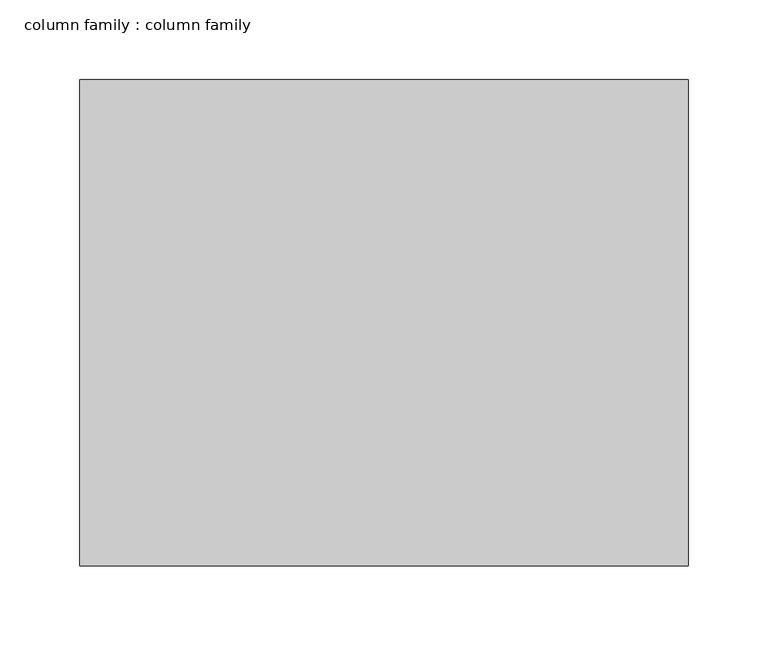
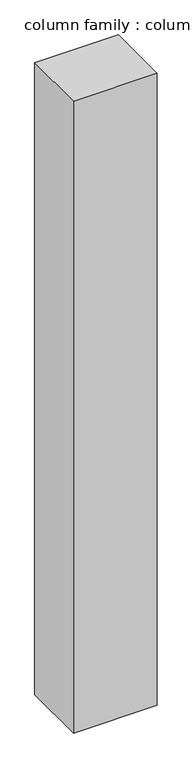
"""IFC4 building model written with IfcOpenShell, lengths in millimetres: column geometry, column family : column family."""

from ifc_helpers import new_model, si_unit, frame, origin, place, context, project, spatial, polyline, outline, extrude, source, transform, mapped, element, save


def column_family_column_family_39b5c8c6(model_context):
    return source(origin(), model_context, "Body", "SweptSolid", [
        extrude(outline(polyline([(246.1278467, 152.4), (246.1278467, -152.4), (-134.8721533, -152.4), (-134.8721533, 152.4), (246.1278467, 152.4)])), frame((0.0, 0.0, 6101.0), z_axis=(0.0, 0.0, 1.0), x_axis=(1.0, 0.0, 0.0)), (0.0, 0.0, 1.0), 3038.0),
    ])


if __name__ == "__main__":
    model = new_model("IFC4")
    model_context = context("Model", 3, world=origin())
    ifc_project = project(units=[si_unit("LENGTHUNIT", "METRE", prefix="MILLI")], contexts=[model_context])
    site = spatial("IfcSite", under=ifc_project)
    building = spatial("IfcBuilding", under=site)
    placement = place(None, origin())
    column_family_column_family_shape = column_family_column_family_39b5c8c6(model_context)
    element("IfcColumn", 1, ObjectType="column family : column family", at=placement, inside=building, context=model_context, shape_type="MappedRepresentation", body=[
        mapped(column_family_column_family_shape, transform((0.0, 0.0, 0.0), x_axis=(1.0, 0.0, 0.0), y_axis=(0.0, 1.0, 0.0), z_axis=(0.0, 0.0, 1.0))),
    ])
    save(model, "model.ifc")

# Revit data of these elements
# Type "column family : column family"
#   w2 [instance default] = 0' - 9.88189"
#   w1 [instance default] = 0' - 9.01575"
#   Depth = 1' - 11.62205"
#   Width = 1' - 11.62205"
# Element 1 (IfcColumn, "column family : column family")
#   w2 = 1' - 0"
#   w1 = 1' - 3"
